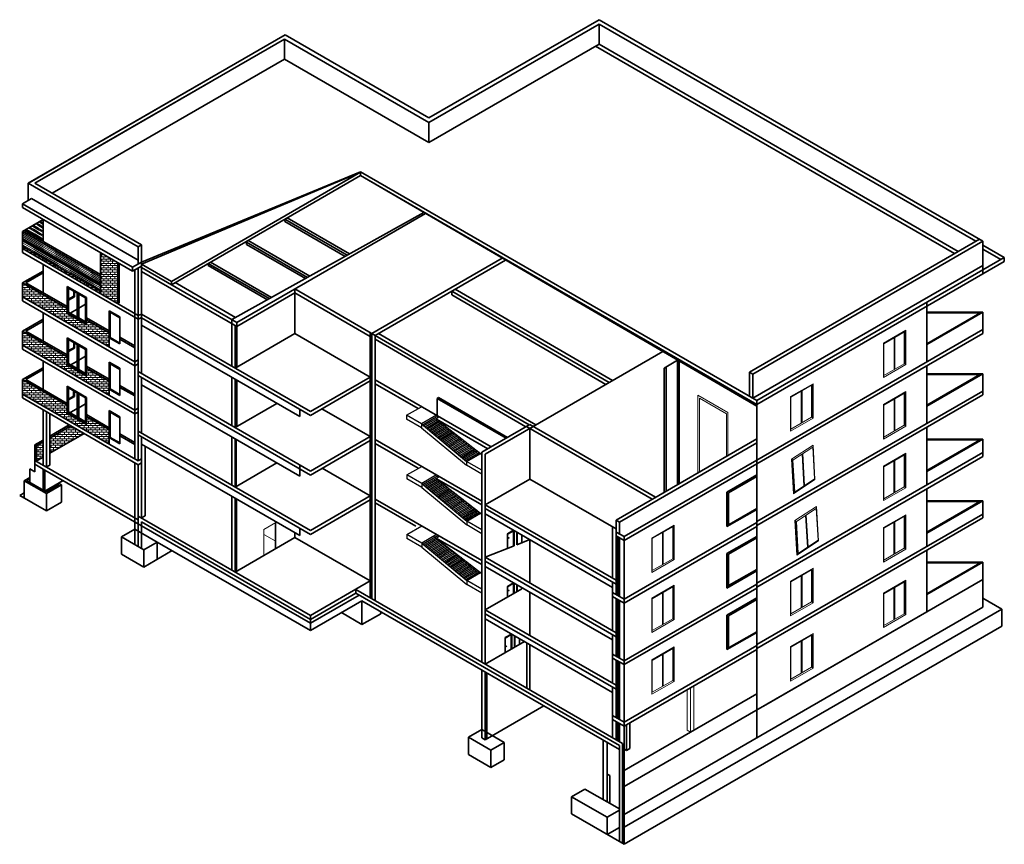
# Model space of a CAD drawing. Units: metres. Extents: x 6326 to 12764, y 4147 to 8354.
# Tile 1 of 2: x 6326 to 6383, y 4147 to 4195. Entities that reach past the tile are written whole.
import ezdxf

# ---------------------------------------------------------------- set-up
doc = ezdxf.new("R2010")
doc.units = ezdxf.units.M
for name, color, linetype, lineweight in [('A-CONS', 9, 'Continuous', 13), ('A-DOOR', 3, 'Continuous', 18), ('A-FLOR-STRS', 3, 'Continuous', 25), ('A-GLAZ', 4, 'Continuous', 18), ('A-SECT', 7, 'Continuous', 35), ('A-WALL-PATT', 8, 'Continuous', 13)]:
    doc.layers.add(name, color=color, linetype=linetype, lineweight=lineweight)

# ---------------------------------------------------------------- blocks, each defined once
blk = doc.blocks.new('tarir')
for p, q in [((6348.756, 4168.452), (6349.622, 4168.952)), ((6349.622, 4167.952), (6348.756, 4168.452)), ((6348.756, 4168.452), (6348.756, 4168.226)), ((6349.622, 4167.726), (6348.756, 4168.226)), ((6350.488, 4168.452), (6349.622, 4167.952)), ((6350.575, 4168.402), (6349.709, 4167.902)), ((6350.575, 4168.302), (6349.764, 4167.834)), ((6350.575, 4168.302), (6349.764, 4167.834)), ((6350.543, 4168.184), (6349.851, 4167.784)), ((6350.488, 4168.252), (6350.488, 4168.152)), ((6350.488, 4168.226), (6353.107, 4166.189)), ((6350.575, 4168.402), (6350.575, 4168.302)), ((6349.622, 4167.952), (6349.622, 4167.726)), ((6349.622, 4167.952), (6352.23, 4165.783)), ((6349.622, 4167.952), (6349.709, 4167.902)), ((6349.622, 4167.726), (6352.23, 4165.557)), ((6349.709, 4167.902), (6349.709, 4167.88)), ((6349.764, 4167.834), (6349.851, 4167.784)), ((6349.851, 4167.784), (6349.851, 4167.762)), ((6350.617, 4168.127), (6349.906, 4167.716)), ((6350.617, 4168.127), (6349.906, 4167.716)), ((6349.906, 4167.716), (6349.993, 4167.666)), ((6350.69, 4168.069), (6349.993, 4167.666)), ((6349.993, 4167.666), (6349.993, 4167.644)), ((6350.764, 4168.012), (6350.048, 4167.598)), ((6350.764, 4168.012), (6350.048, 4167.598)), ((6350.048, 4167.598), (6350.135, 4167.548)), ((6350.838, 4167.954), (6350.135, 4167.548)), ((6350.914, 4167.898), (6350.19, 4167.48)), ((6350.914, 4167.898), (6350.19, 4167.48)), ((6350.986, 4167.84), (6350.276, 4167.43)), ((6351.059, 4167.782), (6350.332, 4167.362)), ((6351.059, 4167.782), (6350.332, 4167.362)), ((6351.133, 4167.725), (6350.418, 4167.312)), ((6351.207, 4167.667), (6350.474, 4167.244)), ((6351.207, 4167.667), (6350.474, 4167.244)), ((6351.281, 4167.61), (6350.56, 4167.194)), ((6350.617, 4168.127), (6350.617, 4168.027)), ((6350.764, 4168.012), (6350.764, 4167.912)), ((6350.912, 4167.897), (6350.912, 4167.797)), ((6351.056, 4167.78), (6351.056, 4167.68)), ((6351.198, 4167.662), (6351.198, 4167.562)), ((6350.135, 4167.548), (6350.135, 4167.526)), ((6350.19, 4167.48), (6350.276, 4167.43)), ((6350.276, 4167.43), (6350.276, 4167.408)), ((6350.332, 4167.362), (6350.418, 4167.312)), ((6350.418, 4167.312), (6350.418, 4167.29)), ((6350.474, 4167.244), (6350.56, 4167.194)), ((6350.56, 4167.194), (6350.56, 4167.172)), ((6351.354, 4167.553), (6350.616, 4167.126)), ((6351.354, 4167.553), (6350.616, 4167.126)), ((6350.616, 4167.126), (6350.702, 4167.076)), ((6351.428, 4167.495), (6350.702, 4167.076)), ((6350.702, 4167.076), (6350.702, 4167.054)), ((6351.502, 4167.438), (6350.757, 4167.008)), ((6351.502, 4167.438), (6350.757, 4167.008)), ((6350.757, 4167.008), (6350.844, 4166.958)), ((6351.576, 4167.38), (6350.844, 4166.958)), ((6351.65, 4167.323), (6350.899, 4166.89)), ((6351.723, 4167.266), (6350.986, 4166.84)), ((6351.797, 4167.208), (6351.041, 4166.772)), ((6351.871, 4167.151), (6351.128, 4166.722)), ((6351.945, 4167.093), (6351.183, 4166.654)), ((6351.945, 4167.093), (6351.183, 4166.654)), ((6352.018, 4167.036), (6351.27, 4166.604)), ((6351.34, 4167.544), (6351.34, 4167.444)), ((6351.482, 4167.426), (6351.482, 4167.326)), ((6351.65, 4167.323), (6351.65, 4167.223)), ((6351.765, 4167.19), (6351.765, 4167.09)), ((6351.907, 4167.072), (6351.907, 4166.972)), ((6350.844, 4166.958), (6350.844, 4166.936)), ((6350.899, 4166.89), (6350.986, 4166.84)), ((6350.986, 4166.84), (6350.986, 4166.818)), ((6351.041, 4166.772), (6351.128, 4166.722)), ((6351.128, 4166.722), (6351.128, 4166.7)), ((6351.183, 4166.654), (6351.27, 4166.604)), ((6351.27, 4166.604), (6351.27, 4166.582)), ((6352.092, 4166.978), (6351.325, 4166.536)), ((6352.092, 4166.978), (6351.325, 4166.536)), ((6351.325, 4166.536), (6351.412, 4166.486)), ((6352.166, 4166.921), (6351.412, 4166.486)), ((6351.412, 4166.486), (6351.412, 4166.463)), ((6352.24, 4166.864), (6351.467, 4166.417)), ((6352.24, 4166.864), (6351.467, 4166.417)), ((6352.314, 4166.806), (6351.554, 4166.367)), ((6352.387, 4166.749), (6351.609, 4166.299)), ((6352.387, 4166.749), (6351.609, 4166.299)), ((6352.461, 4166.691), (6351.695, 4166.249)), ((6352.535, 4166.634), (6351.751, 4166.181)), ((6352.535, 4166.634), (6351.751, 4166.181)), ((6352.609, 4166.577), (6351.837, 4166.131)), ((6352.683, 4166.519), (6351.893, 4166.063)), ((6352.683, 4166.519), (6351.893, 4166.063)), ((6352.756, 4166.462), (6351.979, 4166.013)), ((6352.049, 4166.954), (6352.049, 4166.854)), ((6352.191, 4166.836), (6352.191, 4166.736)), ((6352.333, 4166.717), (6352.333, 4166.617)), ((6352.475, 4166.599), (6352.475, 4166.499)), ((6352.617, 4166.481), (6352.617, 4166.381)), ((6351.467, 4166.417), (6351.554, 4166.367)), ((6351.554, 4166.367), (6351.554, 4166.345)), ((6351.609, 4166.299), (6351.695, 4166.249)), ((6351.695, 4166.249), (6351.695, 4166.227)), ((6351.751, 4166.181), (6351.837, 4166.131)), ((6351.837, 4166.131), (6351.837, 4166.109)), ((6351.893, 4166.063), (6351.979, 4166.013)), ((6351.979, 4166.013), (6351.979, 4165.991)), ((6352.83, 4166.404), (6352.035, 4165.945)), ((6352.035, 4165.945), (6352.121, 4165.895)), ((6352.904, 4166.347), (6352.121, 4165.895)), ((6352.121, 4165.895), (6352.121, 4165.873)), ((6352.978, 4166.29), (6352.176, 4165.827)), ((6352.759, 4166.363), (6352.759, 4166.263)), ((6352.901, 4166.245), (6352.901, 4166.17)), ((6353.107, 4165.276), (6352.23, 4165.783)), ((6352.23, 4165.783), (6352.23, 4165.557)), ((6353.107, 4165.05), (6352.23, 4165.557))]:
    blk.add_line(p, q)
blk = doc.blocks.new('WIN-SINGLE')
for p, q in [((0, 2), (1.299, 2.75)), ((0.022, 1.963), (1.256, 2.675)), ((0.617, 2.306), (0.617, 0.456)), ((0.661, 2.331), (0.661, 0.481)), ((1.213, 2.65), (1.213, 0.8)), ((1.256, 2.675), (1.256, 0.775)), ((1.299, 2.75), (1.299, 0.75)), ((0, 0), (0, 2)), ((0.022, 0.113), (0.022, 1.963)), ((1.299, 0.75), (0, 0)), ((1.213, 0.8), (0.022, 0.113)), ((1.299, 0.75), (1.213, 0.8))]:
    blk.add_line(p, q)
blk = doc.blocks.new('WIN-DOUBLE')
for p, q in [((0, 5.565), (1.299, 6.315)), ((1.299, 6.315), (1.299, 4.315)), ((0.021, 5.528), (1.255, 6.24)), ((0.617, 5.872), (0.617, 4.022)), ((0.66, 5.897), (0.66, 4.047)), ((1.212, 6.215), (1.212, 4.365)), ((1.255, 6.24), (1.255, 4.34)), ((0, 3.565), (0, 5.565)), ((0.021, 3.678), (0.021, 5.528)), ((1.299, 4.315), (0, 3.565)), ((1.212, 4.365), (0.021, 3.678)), ((1.299, 4.315), (1.212, 4.365)), ((0, 2), (1.299, 2.75)), ((0.021, 1.963), (1.255, 2.675)), ((0.617, 2.307), (0.617, 0.457)), ((0.66, 2.332), (0.66, 0.482)), ((1.212, 2.65), (1.212, 0.8)), ((1.255, 2.675), (1.255, 0.775)), ((1.299, 2.75), (1.299, 0.75)), ((0, 0), (0, 2)), ((0.021, 0.113), (0.021, 1.963)), ((1.299, 0.75), (0, 0)), ((1.212, 0.8), (0.021, 0.113)), ((1.299, 0.75), (1.212, 0.8))]:
    blk.add_line(p, q)

msp = doc.modelspace()

# ---------------------------------------------------------------- hatches: boundary and pattern name
at = {"layer": 'A-WALL-PATT'}
h = msp.add_hatch(dxfattribs=at)
h.set_pattern_fill('GOST_GROUND', color=256, scale=0.02, angle=105)
h.paths.add_polyline_path([(6327.679, 4183.255), (6326.587, 4182.625), (6327.679, 4181.995)])
h = msp.add_hatch(dxfattribs=at)
h.set_pattern_fill('GOST_GROUND', color=256, scale=0.04, angle=105)
h.set_pattern_definition([(150, (9e-13, -0.0107), (-0.146410162, 0.546410162), [0.8]), (150, (-0.03106, 0.1052), (-0.146410162, 0.546410162), [0.8]), (150, (-0.0621, 0.2211), (-0.146410162, 0.546410162), [0.8])])
h.paths.add_polyline_path([(6326.489, 4182.558), (6326.489, 4181.708), (6331.012, 4179.107), (6331.012, 4179.946)])
h = msp.add_hatch(dxfattribs=at)
h.set_pattern_fill('BRICK', color=256, scale=0.02, angle=180)
h.paths.add_polyline_path([(6326.489, 4181.713), (6326.489, 4181.568), (6331.012, 4178.957), (6331.012, 4179.102)])
h = msp.add_hatch(dxfattribs=at)
h.set_pattern_fill('BRICK', color=256, scale=0.02, angle=180)
h.paths.add_polyline_path([(6332.018, 4180.752), (6331.012, 4181.333), (6331.012, 4178.957), (6332.018, 4178.376)])
h = msp.add_hatch(dxfattribs=at)
h.set_pattern_fill('GOST_GROUND', color=256, scale=0.1, angle=105)
h.paths.add_polyline_path([(6332.095, 4180.708), (6332.018, 4180.752), (6332.018, 4178.376), (6332.095, 4178.421)])
h = msp.add_hatch(dxfattribs=at)
h.set_pattern_fill('BRICK', color=256, scale=0.02, angle=180)
h.paths.add_polyline_path([(6330.19, 4177.449), (6330.19, 4177.17), (6329.072, 4177.816), (6329.072, 4178.094), (6326.489, 4179.586), (6326.489, 4178.768), (6331.513, 4175.867), (6331.513, 4176.406), (6331.513, 4176.685)])
h = msp.add_hatch(dxfattribs=at)
h.set_pattern_fill('BRICK', color=256, scale=0.02, angle=180)
h.paths.add_polyline_path([(6331.513, 4173.067), (6331.513, 4173.423), (6331.513, 4173.885), (6330.19, 4174.649), (6330.19, 4174.188), (6329.072, 4174.833), (6329.072, 4175.294), (6326.489, 4176.786), (6326.489, 4175.968)])
h = msp.add_hatch(dxfattribs=at)
h.set_pattern_fill('BRICK', color=256, scale=0.02, angle=180)
h.paths.add_polyline_path([(6331.513, 4171.081), (6330.19, 4171.845), (6330.19, 4171.384), (6329.072, 4172.03), (6329.072, 4172.491), (6326.489, 4173.982), (6326.489, 4173.142), (6331.513, 4170.241), (6331.513, 4170.62)])
h = msp.add_hatch(dxfattribs=at)
h.set_pattern_fill('BRICK', color=256, scale=0.02, angle=180)
h.paths.add_polyline_path([(6330.054, 4170.858), (6329.294, 4171.297), (6328.07, 4170.59), (6328.07, 4169.712)])
h = msp.add_hatch(dxfattribs=at)
h.set_pattern_fill('BRICK', color=256, scale=0.02, angle=180)
h.paths.add_polyline_path([(6327.679, 4170.364), (6327.302, 4170.147), (6327.302, 4169.269), (6327.679, 4169.486)])

# ---------------------------------------------------------------- linework, layer by layer
at = {"layer": 'A-CONS'}
for p in [(6353.303, 4163.571), (6353.303, 4160.527)]:
    msp.add_point(p, dxfattribs=at)
at = {"layer": 'A-DOOR'}
for p, q in [((6365.633, 4173.08), (6365.633, 4168.578)), ((6365.633, 4173.08), (6367.365, 4172.08)), ((6365.726, 4172.899), (6365.726, 4168.632)), ((6365.726, 4172.899), (6367.287, 4171.998)), ((6367.287, 4171.998), (6367.287, 4169.533)), ((6367.365, 4172.08), (6367.365, 4169.578)), ((6340.478, 4165.294), (6341.171, 4165.694)), ((6340.478, 4163.794), (6340.478, 4165.294)), ((6341.122, 4165.665), (6341.122, 4164.222)), ((6341.171, 4165.694), (6341.171, 4164.194)), ((6341.122, 4164.627), (6340.478, 4164.998)), ((6341.171, 4164.194), (6341.122, 4164.222))]:
    msp.add_line(p, q, dxfattribs=at)
at = {"layer": 'A-FLOR-STRS'}
for centre in [(6354.659, 4164.803), (6354.659, 4161.759), (6354.524, 4158.524)]:
    msp.add_circle(centre, 0.0242, dxfattribs=at)
at = {"layer": 'A-GLAZ'}
for p, q in [((6362.958, 4161.319), (6364.257, 4162.069)), ((6362.979, 4161.282), (6364.214, 4161.994)), ((6364.17, 4161.969), (6364.17, 4160.119)), ((6364.214, 4161.994), (6364.214, 4160.094)), ((6364.257, 4162.069), (6364.257, 4160.069)), ((6362.958, 4159.319), (6362.958, 4161.319)), ((6363.575, 4161.625), (6363.575, 4159.775)), ((6363.618, 4161.65), (6363.618, 4159.8)), ((6362.979, 4159.432), (6362.979, 4161.282)), ((6364.257, 4160.069), (6362.958, 4159.319)), ((6364.17, 4160.119), (6362.979, 4159.432)), ((6364.257, 4160.069), (6364.17, 4160.119)), ((6362.958, 4157.744), (6364.257, 4158.494)), ((6364.257, 4158.494), (6364.257, 4156.494)), ((6362.979, 4157.707), (6364.214, 4158.419)), ((6363.575, 4158.05), (6363.575, 4156.2)), ((6363.618, 4158.075), (6363.618, 4156.225)), ((6364.17, 4158.394), (6364.17, 4156.544)), ((6364.214, 4158.419), (6364.214, 4156.519)), ((6362.958, 4155.744), (6362.958, 4157.744)), ((6362.979, 4155.857), (6362.979, 4157.707)), ((6364.257, 4156.494), (6362.958, 4155.744)), ((6364.17, 4156.544), (6362.979, 4155.857)), ((6364.257, 4156.494), (6364.17, 4156.544)), ((6365.389, 4156.231), (6365.389, 4153.66)), ((6364.998, 4156.005), (6364.998, 4153.66)), ((6365.193, 4156.118), (6365.193, 4153.547)), ((6365.193, 4153.547), (6364.998, 4153.66))]:
    msp.add_line(p, q, dxfattribs=at)
at = {"layer": 'A-SECT'}
for p, q in [((6350.042, 4189.142), (6359.907, 4194.837)), ((6350.042, 4188.884), (6359.907, 4194.58)), ((6359.907, 4194.837), (6382.141, 4182)), ((6359.907, 4194.58), (6381.736, 4181.993)), ((6359.907, 4194.58), (6359.907, 4193.422)), ((6326.811, 4185.356), (6341.705, 4193.955)), ((6341.705, 4193.955), (6350.043, 4189.141)), ((6327.202, 4185.356), (6341.678, 4193.714)), ((6341.678, 4193.714), (6350.043, 4188.884)), ((6341.678, 4193.714), (6341.678, 4192.556)), ((6350.043, 4187.727), (6359.907, 4193.422)), ((6380.503, 4181.281), (6359.69, 4193.297)), ((6359.907, 4193.422), (6380.72, 4181.406)), ((6328.204, 4184.778), (6341.678, 4192.556)), ((6341.678, 4192.556), (6350.043, 4187.727)), ((6330.038, 4187.219), (6337.226, 4191.369)), ((6330.233, 4187.106), (6337.421, 4191.256)), ((6350.043, 4188.884), (6350.043, 4187.727)), ((6327.006, 4185.469), (6330.038, 4187.219)), ((6327.202, 4185.356), (6330.233, 4187.106)), ((6333.384, 4180.787), (6346.073, 4186.028)), ((6333.384, 4180.674), (6346.073, 4186.002)), ((6335.116, 4179.674), (6346.073, 4186.002)), ((6369.037, 4172.769), (6346.073, 4186.028)), ((6346.073, 4185.802), (6346.073, 4186.028)), ((6326.811, 4185.356), (6327.006, 4185.469)), ((6333.189, 4181.674), (6326.811, 4185.356)), ((6326.811, 4184.356), (6326.811, 4185.356)), ((6333.384, 4181.787), (6327.202, 4185.356)), ((6335.116, 4179.476), (6346.073, 4185.802)), ((6369.037, 4172.543), (6346.073, 4185.802)), ((6369.037, 4172.433), (6346.073, 4185.802)), ((6327.006, 4184.469), (6326.489, 4184.17)), ((6332.866, 4180.488), (6326.489, 4184.17)), ((6326.489, 4183.944), (6326.489, 4184.17)), ((6327.006, 4184.469), (6333.189, 4180.9)), ((6332.866, 4180.262), (6326.489, 4183.944)), ((6338.612, 4177.458), (6349.749, 4183.661)), ((6338.906, 4177.288), (6349.847, 4183.605)), ((6326.489, 4182.568), (6327.68, 4183.256)), ((6327.679, 4181.995), (6327.679, 4183.257)), ((6341.689, 4183.271), (6345.303, 4181.184)), ((6341.689, 4183.271), (6341.689, 4183.142)), ((6341.689, 4183.142), (6345.189, 4181.121)), ((6341.82, 4183.346), (6345.436, 4181.259)), ((6326.489, 4181.342), (6326.489, 4182.568)), ((6326.489, 4181.568), (6326.489, 4182.568)), ((6326.489, 4182.568), (6331.012, 4179.957)), ((6326.587, 4182.625), (6331.012, 4180.07)), ((6326.489, 4182.152), (6331.012, 4179.543)), ((6326.489, 4182.068), (6331.012, 4179.456)), ((6339.469, 4181.989), (6339.469, 4181.815)), ((6339.469, 4181.944), (6343.003, 4179.903)), ((6339.561, 4182.042), (6343.137, 4179.978)), ((6381.945, 4182.113), (6368.611, 4174.415)), ((6382.141, 4182), (6368.807, 4174.302)), ((6382.141, 4182), (6382.141, 4180.109)), ((6326.489, 4181.713), (6331.012, 4179.102)), ((6326.489, 4181.568), (6333.189, 4177.7)), ((6326.489, 4181.342), (6333.189, 4177.474)), ((6331.012, 4181.333), (6331.012, 4178.957)), ((6333.189, 4181.674), (6333.384, 4181.787)), ((6333.189, 4180.674), (6333.189, 4181.674)), ((6333.384, 4180.787), (6333.384, 4181.787)), ((6338.267, 4181.494), (6338.267, 4181.494)), ((6339.469, 4181.815), (6342.89, 4179.84)), ((6383.385, 4181.053), (6382.141, 4181.771)), ((6383.189, 4180.94), (6382.141, 4181.545)), ((6332.018, 4180.752), (6332.018, 4178.376)), ((6332.095, 4180.708), (6332.095, 4178.421)), ((6333.384, 4180.787), (6332.866, 4180.488)), ((6333.384, 4174.327), (6333.384, 4180.787)), ((6337.257, 4180.712), (6340.791, 4178.671)), ((6337.257, 4180.712), (6337.257, 4180.583)), ((6337.388, 4180.788), (6340.925, 4178.746)), ((6346.733, 4176.656), (6354.289, 4181.019)), ((6346.928, 4176.543), (6354.484, 4180.905)), ((6369.037, 4172.769), (6383.385, 4181.053)), ((6369.037, 4172.543), (6383.385, 4180.827)), ((6383.385, 4181.053), (6383.385, 4180.827)), ((6326.489, 4179.586), (6327.679, 4180.273)), ((6326.685, 4179.586), (6327.679, 4180.159)), ((6327.679, 4179.012), (6327.679, 4180.655)), ((6333.384, 4180.561), (6332.866, 4180.262)), ((6332.866, 4180.488), (6332.866, 4180.262)), ((6332.993, 4170.698), (6332.993, 4180.335)), ((6333.189, 4170.585), (6333.189, 4180.448)), ((6333.384, 4180.674), (6335.116, 4179.674)), ((6333.384, 4180.476), (6338.906, 4177.288)), ((6333.384, 4180.25), (6338.906, 4177.062)), ((6336.596, 4180.528), (6336.596, 4180.528)), ((6337.257, 4180.583), (6340.678, 4178.608)), ((6382.141, 4180.6), (6368.807, 4172.902)), ((6382.141, 4180.335), (6382.141, 4180.109)), ((6326.489, 4179.586), (6329.072, 4178.094)), ((6326.489, 4178.542), (6326.489, 4179.586)), ((6326.685, 4179.586), (6329.072, 4178.208)), ((6335.116, 4179.674), (6335.116, 4179.476)), ((6335.335, 4179.602), (6338.835, 4177.581)), ((6329.072, 4177.816), (6329.072, 4179.384)), ((6329.072, 4179.384), (6330.19, 4178.738)), ((6329.158, 4179.284), (6330.146, 4178.713)), ((6329.158, 4177.816), (6329.158, 4179.284)), ((6329.454, 4178.81), (6329.454, 4179.113)), ((6329.497, 4178.785), (6329.497, 4179.088)), ((6329.652, 4178.999), (6329.652, 4177.531)), ((6338.906, 4177.062), (6342.272, 4179.005)), ((6342.272, 4176.649), (6342.272, 4179.231)), ((6342.272, 4179.231), (6346.928, 4176.543)), ((6342.272, 4179.005), (6346.634, 4176.487)), ((6360.485, 4173.806), (6351.374, 4179.11)), ((6351.374, 4179.11), (6351.374, 4178.884)), ((6360.681, 4173.919), (6351.57, 4179.223)), ((6326.489, 4178.742), (6326.489, 4178.968)), ((6326.489, 4178.768), (6332.993, 4175.013)), ((6326.489, 4178.542), (6332.993, 4174.787)), ((6329.158, 4178.639), (6329.454, 4178.81)), ((6329.158, 4178.589), (6329.497, 4178.785)), ((6329.68, 4178.983), (6329.68, 4177.514)), ((6329.746, 4178.945), (6329.746, 4177.552)), ((6330.146, 4178.713), (6330.146, 4177.245)), ((6330.19, 4178.738), (6330.19, 4177.17)), ((6332.018, 4178.376), (6332.095, 4178.421)), ((6360.29, 4173.693), (6351.374, 4178.884)), ((6378.89, 4178.458), (6378.89, 4175.006)), ((6327.679, 4176.212), (6327.679, 4177.855)), ((6329.652, 4177.606), (6329.158, 4177.892)), ((6329.258, 4177.834), (6329.652, 4178.062)), ((6329.746, 4178.116), (6330.146, 4178.347)), ((6331.513, 4176.406), (6331.513, 4177.974)), ((6331.513, 4177.974), (6332.134, 4177.616)), ((6331.563, 4176.419), (6331.563, 4177.879)), ((6331.563, 4177.879), (6332.121, 4177.557)), ((6378.89, 4177.891), (6382.141, 4177.883)), ((6382.141, 4177.883), (6378.89, 4176.006)), ((6382.141, 4177.883), (6382.141, 4176.883)), ((6382.141, 4177.883), (6382.141, 4176.656)), ((6326.489, 4176.786), (6327.679, 4177.473)), ((6326.685, 4176.786), (6327.679, 4177.359)), ((6329.072, 4177.816), (6330.19, 4177.17)), ((6329.158, 4177.816), (6330.146, 4177.245)), ((6329.68, 4177.514), (6329.746, 4177.552)), ((6329.746, 4177.552), (6330.146, 4177.321)), ((6330.19, 4177.562), (6331.513, 4176.798)), ((6330.19, 4177.449), (6331.513, 4176.685)), ((6332.121, 4176.097), (6332.121, 4177.557)), ((6332.134, 4176.048), (6332.134, 4177.616)), ((6333.384, 4177.78), (6333.189, 4177.7)), ((6333.189, 4177.474), (6333.384, 4177.587)), ((6333.384, 4177.78), (6343.17, 4172.13)), ((6333.384, 4177.553), (6343.17, 4171.903)), ((6338.612, 4177.232), (6338.612, 4177.458)), ((6338.906, 4174.705), (6338.906, 4177.288)), ((6378.89, 4177.841), (6381.969, 4177.834)), ((6381.969, 4177.834), (6378.89, 4176.056)), ((6326.489, 4176.786), (6329.072, 4175.294)), ((6326.489, 4175.742), (6326.489, 4176.786)), ((6326.685, 4176.786), (6329.072, 4175.408)), ((6333.384, 4177.127), (6342.554, 4171.833)), ((6338.612, 4174.762), (6338.612, 4177.232)), ((6338.808, 4174.649), (6338.808, 4177.119)), ((6346.634, 4161.333), (6346.634, 4176.713)), ((6382.141, 4176.883), (6369.037, 4169.318)), ((6326.489, 4175.942), (6326.489, 4176.168)), ((6329.072, 4174.833), (6329.072, 4176.401)), ((6329.072, 4176.401), (6330.19, 4175.756)), ((6329.158, 4176.301), (6330.146, 4175.731)), ((6329.158, 4174.833), (6329.158, 4176.301)), ((6331.513, 4176.406), (6332.134, 4176.048)), ((6331.513, 4176.406), (6331.513, 4175.867)), ((6331.563, 4176.419), (6332.121, 4176.097)), ((6332.134, 4176.44), (6332.993, 4175.944)), ((6332.134, 4176.326), (6332.993, 4175.83)), ((6338.808, 4174.649), (6342.272, 4176.649)), ((6346.634, 4174.13), (6342.272, 4176.649)), ((6346.733, 4161.276), (6346.733, 4176.656)), ((6346.928, 4161.163), (6346.928, 4176.543)), ((6355.845, 4171.352), (6346.928, 4176.543)), ((6346.928, 4176.543), (6346.928, 4176.317)), ((6355.65, 4171.24), (6346.928, 4176.317)), ((6356.235, 4171.352), (6347.124, 4176.656)), ((6382.141, 4176.656), (6369.037, 4169.091)), ((6326.489, 4175.968), (6332.993, 4172.213)), ((6326.489, 4175.742), (6332.993, 4171.987)), ((6329.16, 4175.657), (6329.454, 4175.827)), ((6329.16, 4175.607), (6329.497, 4175.802)), ((6329.454, 4175.827), (6329.454, 4176.13)), ((6329.497, 4175.802), (6329.497, 4176.105)), ((6329.652, 4176.016), (6329.652, 4174.548)), ((6329.68, 4176), (6329.68, 4174.532)), ((6329.746, 4175.962), (6329.746, 4174.57)), ((6330.146, 4175.731), (6330.146, 4174.263)), ((6330.19, 4175.756), (6330.19, 4174.188)), ((6356.077, 4171.261), (6363.595, 4175.601)), ((6327.679, 4173.409), (6327.679, 4175.055)), ((6329.28, 4174.838), (6329.652, 4175.053)), ((6329.746, 4175.107), (6330.146, 4175.338)), ((6332.993, 4175.013), (6333.189, 4175.126)), ((6364.454, 4175.101), (6363.665, 4174.645)), ((6364.454, 4175.101), (6364.454, 4167.898)), ((6364.548, 4175.047), (6364.548, 4167.952)), ((6326.489, 4173.982), (6327.679, 4174.669)), ((6326.685, 4173.982), (6327.679, 4174.556)), ((6329.072, 4174.833), (6330.19, 4174.188)), ((6329.652, 4174.624), (6329.158, 4174.909)), ((6329.158, 4174.833), (6330.146, 4174.263)), ((6329.68, 4174.532), (6329.746, 4174.57)), ((6329.746, 4174.57), (6330.146, 4174.338)), ((6330.19, 4174.762), (6331.513, 4173.998)), ((6330.19, 4174.649), (6331.513, 4173.885)), ((6331.513, 4173.423), (6331.513, 4174.991)), ((6331.513, 4174.991), (6332.134, 4174.633)), ((6331.563, 4173.436), (6331.563, 4174.896)), ((6331.563, 4174.896), (6332.121, 4174.574)), ((6332.121, 4173.114), (6332.121, 4174.574)), ((6332.134, 4173.065), (6332.134, 4174.633)), ((6332.993, 4174.787), (6333.189, 4174.9)), ((6333.189, 4174.44), (6343.17, 4168.677)), ((6363.665, 4174.645), (6363.665, 4167.442)), ((6363.785, 4174.715), (6363.785, 4167.511)), ((6378.89, 4174.779), (6378.89, 4171.441)), ((6326.489, 4173.982), (6329.072, 4172.491)), ((6326.489, 4172.916), (6326.489, 4173.982)), ((6326.685, 4173.982), (6329.072, 4172.604)), ((6333.189, 4174.214), (6343.17, 4168.451)), ((6333.384, 4170.888), (6333.384, 4174.101)), ((6338.612, 4171.309), (6338.612, 4174.109)), ((6338.808, 4171.196), (6338.808, 4173.996)), ((6338.906, 4171.253), (6338.906, 4173.939)), ((6343.17, 4172.13), (6346.634, 4174.13)), ((6343.17, 4171.903), (6346.634, 4173.903)), ((6346.928, 4173.96), (6353.645, 4170.083)), ((6365.726, 4174.361), (6365.726, 4174.361)), ((6368.807, 4174.302), (6368.611, 4174.415)), ((6368.612, 4174.415), (6368.612, 4173.015)), ((6368.807, 4174.302), (6368.807, 4172.902)), ((6378.89, 4174.326), (6382.141, 4174.318)), ((6382.141, 4174.318), (6378.89, 4172.441)), ((6378.89, 4174.276), (6381.969, 4174.269)), ((6381.969, 4174.269), (6378.89, 4172.491)), ((6382.141, 4174.318), (6382.141, 4173.318)), ((6382.141, 4174.318), (6382.141, 4173.091)), ((6329.072, 4172.03), (6329.072, 4173.598)), ((6329.072, 4173.598), (6330.19, 4172.952)), ((6329.158, 4173.498), (6330.146, 4172.927)), ((6329.158, 4172.03), (6329.158, 4173.498)), ((6329.452, 4173.025), (6329.452, 4173.328)), ((6329.496, 4173), (6329.496, 4173.303)), ((6331.513, 4173.423), (6332.134, 4173.065)), ((6331.513, 4173.423), (6331.513, 4173.067)), ((6331.563, 4173.436), (6332.121, 4173.114)), ((6332.134, 4173.64), (6332.993, 4173.144)), ((6332.134, 4173.526), (6332.993, 4173.03)), ((6333.384, 4173.675), (6342.554, 4168.381)), ((6346.928, 4173.734), (6349.416, 4172.297)), ((6367.365, 4173.415), (6367.365, 4173.407)), ((6382.141, 4173.318), (6369.037, 4165.753)), ((6326.489, 4173.142), (6333.189, 4169.274)), ((6326.489, 4172.916), (6333.189, 4169.048)), ((6329.158, 4172.855), (6329.452, 4173.025)), ((6329.158, 4172.805), (6329.496, 4173)), ((6329.652, 4173.212), (6329.652, 4171.744)), ((6329.68, 4173.196), (6329.68, 4171.728)), ((6329.746, 4173.158), (6329.746, 4171.766)), ((6330.146, 4172.927), (6330.146, 4171.459)), ((6330.19, 4172.952), (6330.19, 4171.384)), ((6350.517, 4172.889), (6350.603, 4172.939)), ((6354.511, 4170.583), (6350.517, 4172.889)), ((6350.517, 4172.889), (6350.517, 4171.889)), ((6354.598, 4170.633), (6350.603, 4172.939)), ((6382.141, 4173.091), (6369.037, 4165.526)), ((6369.037, 4172.769), (6369.037, 4153.217)), ((6327.679, 4169.029), (6327.679, 4172.229)), ((6329.238, 4172.059), (6329.652, 4172.298)), ((6329.746, 4172.352), (6330.146, 4172.583)), ((6331.513, 4170.62), (6331.513, 4172.188)), ((6331.513, 4172.188), (6332.134, 4171.83)), ((6332.993, 4172.213), (6333.189, 4172.326)), ((6338.808, 4171.196), (6341.233, 4172.596)), ((6342.554, 4171.833), (6342.554, 4172.259)), ((6346.634, 4170.677), (6343.841, 4172.29)), ((6327.874, 4168.916), (6327.874, 4172.116)), ((6328.07, 4169.029), (6328.07, 4172.003)), ((6329.072, 4172.03), (6330.19, 4171.384)), ((6329.652, 4171.82), (6329.158, 4172.105)), ((6329.158, 4172.03), (6330.146, 4171.459)), ((6329.68, 4171.728), (6329.746, 4171.766)), ((6329.746, 4171.766), (6330.146, 4171.535)), ((6330.19, 4171.959), (6331.513, 4171.194)), ((6330.19, 4171.845), (6331.513, 4171.081)), ((6331.563, 4170.632), (6331.563, 4172.093)), ((6331.563, 4172.093), (6332.121, 4171.771)), ((6332.121, 4170.311), (6332.121, 4171.771)), ((6332.134, 4170.261), (6332.134, 4171.83)), ((6332.993, 4171.987), (6333.189, 4172.1)), ((6350.479, 4171.684), (6353.449, 4169.969)), ((6328.07, 4170.699), (6329.2, 4171.351)), ((6328.07, 4170.59), (6329.294, 4171.297)), ((6332.993, 4169.387), (6332.993, 4171.387)), ((6333.189, 4169.274), (6333.189, 4171.274)), ((6333.189, 4171.001), (6343.17, 4165.238)), ((6353.107, 4169.772), (6355.882, 4171.374)), ((6353.303, 4169.659), (6356.077, 4171.261)), ((6355.686, 4171.261), (6362.983, 4167.048)), ((6355.882, 4171.374), (6363.178, 4167.161)), ((6355.882, 4171.148), (6355.882, 4168.217)), ((6378.89, 4171.214), (6378.89, 4167.876)), ((6327.208, 4170.201), (6327.679, 4170.473)), ((6328.07, 4169.712), (6330.054, 4170.858)), ((6331.513, 4170.62), (6332.134, 4170.261)), ((6331.513, 4170.62), (6331.513, 4170.241)), ((6331.563, 4170.632), (6332.121, 4170.311)), ((6332.134, 4170.836), (6332.993, 4170.34)), ((6332.134, 4170.723), (6332.993, 4170.227)), ((6333.189, 4170.774), (6343.17, 4165.011)), ((6333.384, 4169.161), (6333.384, 4170.661)), ((6338.612, 4167.869), (6338.612, 4170.656)), ((6338.808, 4167.756), (6338.808, 4170.543)), ((6338.865, 4167.789), (6338.865, 4170.51)), ((6343.17, 4168.677), (6346.634, 4170.677)), ((6343.17, 4168.451), (6346.634, 4170.451)), ((6346.928, 4170.508), (6353.107, 4166.941)), ((6360.884, 4165.836), (6369.037, 4170.544)), ((6378.89, 4170.534), (6382.141, 4170.526)), ((6382.141, 4170.526), (6378.89, 4168.649)), ((6378.89, 4170.484), (6381.952, 4170.477)), ((6381.952, 4170.477), (6378.89, 4168.709)), ((6382.141, 4170.526), (6382.141, 4169.753)), ((6382.141, 4170.526), (6382.141, 4169.526)), ((6327.208, 4169.301), (6327.208, 4170.201)), ((6327.302, 4170.147), (6327.208, 4170.201)), ((6327.302, 4170.147), (6327.679, 4170.364)), ((6327.302, 4169.247), (6327.302, 4170.147)), ((6333.384, 4170.235), (6342.554, 4164.941)), ((6333.593, 4166.082), (6333.593, 4170.115)), ((6346.928, 4170.282), (6349.426, 4168.839)), ((6369.037, 4170.318), (6361.08, 4165.723)), ((6327.208, 4169.075), (6327.208, 4169.301)), ((6327.208, 4169.301), (6333.189, 4165.848)), ((6327.283, 4169.258), (6327.679, 4169.486)), ((6333.189, 4169.274), (6333.384, 4169.387)), ((6352.22, 4169.241), (6353.024, 4169.705)), ((6353.107, 4169.772), (6353.107, 4157.596)), ((6353.303, 4169.659), (6353.303, 4157.483)), ((6369.037, 4169.318), (6361.349, 4164.879)), ((6382.141, 4169.753), (6369.037, 4162.188)), ((6382.141, 4169.526), (6369.037, 4161.961)), ((6326.912, 4168.022), (6326.912, 4168.814)), ((6326.912, 4168.814), (6327.208, 4168.643)), ((6327.208, 4168.643), (6327.208, 4169.075)), ((6327.208, 4169.075), (6327.792, 4168.738)), ((6327.679, 4167.579), (6327.679, 4168.803)), ((6327.792, 4167.514), (6327.792, 4168.738)), ((6327.792, 4168.738), (6333.384, 4165.509)), ((6327.874, 4168.916), (6328.07, 4169.029)), ((6332.993, 4165.961), (6332.993, 4169.161)), ((6333.189, 4169.048), (6333.384, 4169.161)), ((6333.189, 4164.308), (6333.189, 4169.048)), ((6333.384, 4165.961), (6333.384, 4169.161)), ((6338.808, 4167.756), (6341.221, 4169.15)), ((6342.554, 4168.381), (6342.554, 4169.033)), ((6346.634, 4167.238), (6343.852, 4168.844)), ((6369.037, 4169.092), (6361.349, 4164.653)), ((6326.583, 4168.122), (6326.912, 4168.312)), ((6326.726, 4168.129), (6326.912, 4168.236)), ((6350.488, 4168.226), (6353.107, 4166.715)), ((6353.303, 4166.728), (6355.882, 4168.217)), ((6355.882, 4168.217), (6360.884, 4165.329)), ((6369.037, 4168.461), (6367.314, 4167.466)), ((6369.037, 4168.369), (6367.401, 4167.424)), ((6326.583, 4167.122), (6326.583, 4168.122)), ((6326.583, 4168.122), (6327.878, 4167.375)), ((6326.726, 4168.129), (6327.865, 4167.472)), ((6327.792, 4167.514), (6328.852, 4168.126)), ((6328.603, 4167.898), (6327.865, 4167.472)), ((6328.744, 4167.875), (6327.878, 4167.375)), ((6328.529, 4167.94), (6328.603, 4167.898)), ((6328.58, 4167.969), (6328.744, 4167.875)), ((6328.744, 4166.875), (6328.744, 4167.875)), ((6353.107, 4166.941), (6353.107, 4167.941)), ((6378.89, 4167.649), (6378.89, 4164.311)), ((6326.326, 4167.27), (6326.583, 4167.419)), ((6326.326, 4167.27), (6327.878, 4166.375)), ((6327.878, 4167.375), (6327.878, 4166.375)), ((6338.612, 4162.943), (6338.612, 4167.217)), ((6338.808, 4162.83), (6338.808, 4167.104)), ((6338.897, 4162.901), (6338.897, 4167.052)), ((6343.17, 4165.238), (6346.634, 4167.238)), ((6343.17, 4165.011), (6346.634, 4167.011)), ((6346.928, 4167.058), (6353.107, 4163.491)), ((6367.314, 4167.466), (6367.314, 4165.466)), ((6367.401, 4167.424), (6367.401, 4165.558)), ((6327.878, 4166.375), (6328.744, 4166.875)), ((6346.928, 4166.838), (6349.274, 4165.484)), ((6353.303, 4166.728), (6360.884, 4162.351)), ((6353.303, 4166.501), (6360.884, 4162.124)), ((6367.314, 4165.507), (6369.037, 4166.502)), ((6367.314, 4165.466), (6369.037, 4166.461)), ((6378.89, 4166.969), (6382.141, 4166.961)), ((6382.141, 4166.961), (6378.89, 4165.084)), ((6378.89, 4166.919), (6381.969, 4166.912)), ((6381.969, 4166.912), (6378.89, 4165.134)), ((6382.141, 4166.961), (6382.141, 4166.188)), ((6382.141, 4166.961), (6382.141, 4165.961)), ((6332.993, 4164.421), (6332.993, 4165.961)), ((6333.189, 4166.074), (6343.17, 4160.311)), ((6333.384, 4165.961), (6333.593, 4166.082)), ((6352.23, 4165.783), (6353.033, 4166.246)), ((6353.303, 4166.201), (6360.688, 4161.937)), ((6382.141, 4166.188), (6369.037, 4158.623)), ((6382.141, 4165.961), (6369.037, 4158.396)), ((6332.219, 4164.868), (6332.993, 4165.315)), ((6332.993, 4165.315), (6334.288, 4164.567)), ((6333.384, 4164.195), (6333.384, 4165.735)), ((6333.384, 4165.735), (6343.17, 4160.085)), ((6333.384, 4165.509), (6343.17, 4159.859)), ((6342.554, 4165.367), (6342.554, 4164.941)), ((6360.688, 4162.464), (6360.688, 4165.442)), ((6360.884, 4165.836), (6361.08, 4165.723)), ((6360.884, 4161.523), (6360.884, 4165.836)), ((6361.08, 4165.035), (6361.08, 4165.723)), ((6369.037, 4165.693), (6361.349, 4161.254)), ((6369.037, 4165.467), (6361.349, 4161.028)), ((6332.219, 4163.868), (6332.219, 4164.868)), ((6333.514, 4164.12), (6332.219, 4164.868)), ((6338.808, 4162.83), (6342.272, 4164.83)), ((6342.272, 4164.83), (6342.272, 4165.104)), ((6346.634, 4162.311), (6342.272, 4164.83)), ((6350.331, 4164.873), (6353.107, 4163.271)), ((6354.951, 4165.25), (6354.592, 4165.043)), ((6354.951, 4165.222), (6354.592, 4165.015)), ((6354.592, 4164.198), (6354.592, 4165.043)), ((6354.951, 4164.341), (6354.951, 4165.222)), ((6354.975, 4164.351), (6354.975, 4165.236)), ((6355.134, 4164.414), (6355.134, 4165.144)), ((6355.155, 4164.423), (6355.155, 4165.132)), ((6355.421, 4164.529), (6355.421, 4164.978)), ((6361.349, 4164.879), (6360.884, 4165.148)), ((6361.349, 4164.653), (6360.884, 4164.922)), ((6360.988, 4164.861), (6360.988, 4161.463)), ((6361.08, 4164.809), (6361.08, 4161.41)), ((6361.08, 4164.809), (6361.08, 4161.41)), ((6361.349, 4164.653), (6361.349, 4164.879)), ((6369.037, 4164.896), (6367.314, 4163.901)), ((6369.037, 4164.804), (6367.401, 4163.859)), ((6333.514, 4164.12), (6334.288, 4164.567)), ((6334.288, 4164.567), (6334.288, 4163.567)), ((6334.288, 4164.567), (6343.17, 4159.439)), ((6354.975, 4164.351), (6353.303, 4163.684)), ((6355.882, 4164.712), (6355.134, 4164.414)), ((6355.882, 4164.712), (6355.882, 4162.195)), ((6361.349, 4161.254), (6361.349, 4164.653)), ((6332.219, 4163.868), (6333.514, 4163.12)), ((6332.219, 4163.868), (6333.514, 4163.12)), ((6333.514, 4163.12), (6333.514, 4164.12)), ((6333.514, 4163.12), (6335.154, 4164.067)), ((6353.303, 4163.684), (6360.884, 4159.307)), ((6367.314, 4163.901), (6367.314, 4161.901)), ((6367.401, 4163.859), (6367.401, 4162.039)), ((6378.89, 4164.084), (6378.89, 4160.519)), ((6353.303, 4163.458), (6360.884, 4159.08)), ((6353.303, 4163.158), (6360.688, 4158.893)), ((6378.89, 4163.404), (6382.141, 4163.396)), ((6382.141, 4163.396), (6378.89, 4161.519)), ((6378.89, 4163.354), (6381.969, 4163.347)), ((6381.969, 4163.347), (6378.89, 4161.569)), ((6382.141, 4163.396), (6382.141, 4162.396)), ((6382.141, 4163.396), (6382.141, 4162.51)), ((6352.23, 4162.333), (6353.033, 4162.797)), ((6367.314, 4161.989), (6369.037, 4162.984)), ((6367.314, 4161.901), (6369.037, 4162.896)), ((6382.141, 4162.623), (6382.141, 4162.396)), ((6343.17, 4160.311), (6346.634, 4162.311)), ((6354.951, 4162.206), (6354.592, 4161.999)), ((6354.951, 4162.178), (6354.592, 4161.971)), ((6354.592, 4161.385), (6354.592, 4161.999)), ((6354.951, 4161.592), (6354.951, 4162.178)), ((6354.975, 4161.606), (6354.975, 4162.192)), ((6355.134, 4161.698), (6355.134, 4162.1)), ((6355.155, 4161.71), (6355.155, 4162.088)), ((6355.421, 4161.864), (6355.421, 4161.934)), ((6360.688, 4159.42), (6360.688, 4162.237)), ((6369.037, 4162.128), (6361.349, 4157.689)), ((6369.037, 4161.902), (6361.349, 4157.463)), ((6382.141, 4162.396), (6369.429, 4155.057)), ((6382.141, 4162.396), (6382.141, 4160.783)), ((6343.17, 4160.085), (6345.797, 4161.602)), ((6343.17, 4159.859), (6345.993, 4161.489)), ((6345.797, 4161.602), (6345.797, 4161.828)), ((6345.797, 4161.816), (6353.107, 4157.596)), ((6345.797, 4161.602), (6361.08, 4152.779)), ((6353.303, 4160.64), (6355.421, 4161.864)), ((6355.882, 4161.668), (6355.882, 4159.151)), ((6361.349, 4161.254), (6360.688, 4161.636)), ((6361.349, 4161.028), (6360.688, 4161.41)), ((6369.037, 4161.331), (6367.314, 4160.336)), ((6383.232, 4160.684), (6382.141, 4161.313)), ((6343.17, 4159.439), (6346.161, 4161.166)), ((6346.161, 4161.166), (6361.08, 4152.553)), ((6346.161, 4161.166), (6346.161, 4159.786)), ((6360.884, 4157.958), (6360.884, 4161.297)), ((6360.988, 4161.237), (6360.988, 4157.898)), ((6361.08, 4161.184), (6361.08, 4157.845)), ((6361.08, 4161.184), (6361.08, 4157.845)), ((6361.349, 4154.124), (6361.349, 4161.254)), ((6361.349, 4148.778), (6382.141, 4160.783)), ((6369.037, 4161.239), (6367.401, 4160.294)), ((6343.17, 4160.311), (6343.17, 4159.439)), ((6344.967, 4160.476), (6346.161, 4159.786)), ((6346.161, 4159.786), (6347.249, 4160.414)), ((6347.249, 4160.414), (6347.249, 4160.538)), ((6353.303, 4160.64), (6360.884, 4156.263)), ((6353.303, 4160.414), (6360.884, 4156.036)), ((6361.349, 4148.05), (6383.232, 4160.684)), ((6361.349, 4150.392), (6378.89, 4160.519)), ((6367.314, 4160.336), (6367.314, 4158.336)), ((6367.401, 4160.294), (6367.401, 4158.421)), ((6383.232, 4160.684), (6383.232, 4159.684)), ((6353.303, 4160.114), (6360.688, 4155.849)), ((6361.349, 4147.05), (6383.232, 4159.684)), ((6354.821, 4159.237), (6354.458, 4159.027)), ((6354.816, 4159.206), (6354.458, 4158.999)), ((6354.458, 4158.15), (6354.458, 4159.027)), ((6354.816, 4158.357), (6354.816, 4159.206)), ((6354.841, 4158.371), (6354.841, 4159.226)), ((6354.999, 4158.463), (6354.999, 4159.134)), ((6355.02, 4158.475), (6355.02, 4159.122)), ((6360.688, 4156.376), (6360.688, 4159.193)), ((6367.314, 4158.37), (6369.037, 4159.365)), ((6367.314, 4158.336), (6369.037, 4159.331)), ((6353.303, 4157.483), (6355.581, 4158.798)), ((6355.287, 4158.629), (6355.287, 4158.968)), ((6355.71, 4158.724), (6355.71, 4156.093)), ((6355.882, 4158.625), (6355.882, 4155.994)), ((6369.037, 4158.563), (6361.349, 4154.124)), ((6361.349, 4157.689), (6360.688, 4158.071)), ((6369.037, 4158.337), (6361.349, 4153.898)), ((6353.107, 4157.596), (6361.258, 4152.89)), ((6361.349, 4157.463), (6360.688, 4157.845)), ((6360.884, 4154.393), (6360.884, 4157.732)), ((6360.988, 4157.672), (6360.988, 4154.333)), ((6361.08, 4157.619), (6361.08, 4154.28)), ((6361.08, 4157.619), (6361.08, 4154.28)), ((6353.107, 4157.156), (6353.107, 4153.702)), ((6353.303, 4157.043), (6353.303, 4153.11)), ((6353.303, 4157.043), (6353.303, 4153.11)), ((6353.401, 4156.986), (6353.401, 4153.166)), ((6360.688, 4153.219), (6360.688, 4156.149)), ((6361.349, 4151.328), (6369.037, 4155.767)), ((6353.303, 4153.11), (6356.709, 4155.076)), ((6361.349, 4154.124), (6360.688, 4154.506)), ((6353.107, 4153.223), (6353.107, 4154.348)), ((6361.349, 4153.898), (6360.688, 4154.28)), ((6360.884, 4153.106), (6360.884, 4154.167)), ((6360.988, 4154.107), (6360.988, 4153.046)), ((6361.08, 4154.054), (6361.08, 4152.993)), ((6361.08, 4154.054), (6361.08, 4152.993)), ((6361.349, 4153.898), (6361.349, 4154.124)), ((6361.349, 4153.898), (6361.349, 4147.05)), ((6361.495, 4152.488), (6361.495, 4153.983)), ((6361.691, 4154.096), (6361.691, 4152.601)), ((6352.333, 4153.255), (6353.107, 4153.702)), ((6353.107, 4153.702), (6354.402, 4152.954)), ((6352.333, 4152.255), (6352.333, 4153.255)), ((6352.333, 4153.255), (6353.628, 4152.508)), ((6353.107, 4153.223), (6353.303, 4153.11)), ((6353.628, 4152.508), (6354.402, 4152.954)), ((6354.402, 4152.954), (6354.402, 4151.954)), ((6360.146, 4149.638), (6360.146, 4153.092)), ((6360.373, 4152.96), (6360.373, 4149.506)), ((6361.08, 4152.779), (6361.08, 4152.553)), ((6361.08, 4152.779), (6361.08, 4147.205)), ((6361.258, 4152.89), (6361.258, 4147.103)), ((6352.333, 4152.255), (6353.628, 4151.508)), ((6352.333, 4152.255), (6353.628, 4151.508)), ((6353.628, 4151.508), (6353.628, 4152.508)), ((6361.495, 4152.488), (6361.258, 4152.625)), ((6361.495, 4152.488), (6361.691, 4152.601)), ((6353.628, 4151.508), (6354.402, 4151.954)), ((6360.373, 4151.12), (6360.516, 4151.038)), ((6360.516, 4151.038), (6360.516, 4149.424)), ((6358.305, 4149.807), (6359.079, 4150.254)), ((6359.079, 4150.254), (6361.08, 4149.099)), ((6358.305, 4148.807), (6358.305, 4149.807)), ((6360.373, 4148.613), (6358.305, 4149.807)), ((6358.305, 4148.807), (6361.349, 4147.05)), ((6360.373, 4148.613), (6361.08, 4149.021)), ((6360.373, 4147.613), (6360.373, 4148.613)), ((6360.373, 4148.613), (6360.373, 4148.506)), ((6360.373, 4148.613), (6360.373, 4147.613)), ((6360.373, 4147.613), (6361.08, 4148.021))]:
    msp.add_line(p, q, dxfattribs=at)

# ---------------------------------------------------------------- block references
at = {"layer": 'A-FLOR-STRS'}
for p in [(-0.009, 3.458), (0, 0), (0, -3.45)]:
    msp.add_blockref('tarir', p, dxfattribs=at)
at = {"layer": 'A-GLAZ'}
for name, p in [('WIN-DOUBLE', (6376.376, 4170.532)), ('WIN-SINGLE', (6371, 4170.994)), ('WIN-SINGLE', (6376.375, 4166.967)), ('WIN-SINGLE', (6376.375, 4163.402)), ('WIN-SINGLE', (6362.957, 4162.8)), ('WIN-SINGLE', (6371, 4160.299)), ('WIN-SINGLE', (6376.375, 4159.61)), ('WIN-SINGLE', (6371, 4156.507))]:
    msp.add_blockref(name, p, dxfattribs=at)
at = {"layer": 'A-GLAZ', "rotation": 183.2445806698638}
msp.add_blockref('WIN-DOUBLE', (6372.3, 4170.187), dxfattribs=at)

doc.saveas('drawing.dxf')
